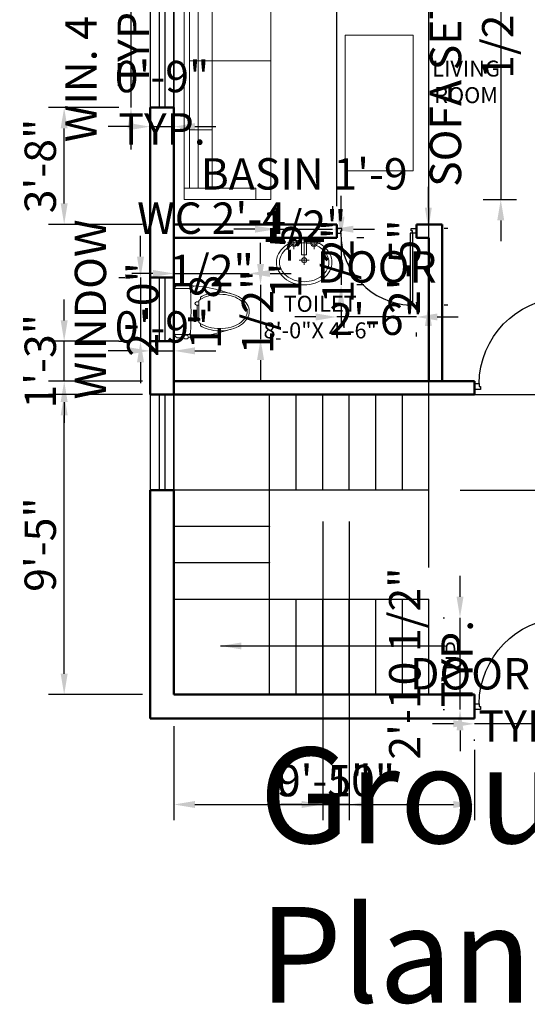
# Model space of a CAD drawing. Units: inches. Extents: x 117606 to 118050, y 251709 to 252357.
# Tile 1 of 3: x 117606 to 117797, y 251709 to 252079. Entities that reach past the tile are written whole.
import ezdxf

# ---------------------------------------------------------------- set-up
doc = ezdxf.new("R2010")
doc.units = ezdxf.units.IN
doc.header["$MEASUREMENT"] = 0
for name, color, linetype, lineweight in [('A-ANNO-SYMB', 7, 'Continuous', 18), ('A-ANNO-TEXT', 7, 'Continuous', 25), ('A-AREA-IDEN', 7, 'Continuous', 25), ('A-DOOR', 4, 'Continuous', 25), ('A-FLOR-CNST', 8, 'Continuous', 13), ('A-FLOR-STRS', 7, 'Continuous', 25), ('FURNITURE', 53, 'Continuous', 18), ('SANITARY', 151, 'Continuous', 18), ('WALL', 7, 'Continuous', 50), ('WINDOW', 2, 'Continuous', 25), ('YQ_DIM', 3, 'Continuous', 18)]:
    doc.layers.add(name, color=color, linetype=linetype, lineweight=lineweight)
doc.styles.add('YQ_DIM', font='SUPEROS.SHX', dxfattribs={"width": 0.8, "bigfont": 'HZDX.SHX'})
doc.dimstyles.new('yqi3_937', dxfattribs={"dimscale": 3.937008, "dimtxt": 3, "dimasz": 2, "dimexe": 1.5, "dimexo": 3, "dimgap": 0.5, "dimtad": 1, "dimdsep": 46, "dimlunit": 4, "dimtxsty": 'YQ_DIM', "dimcen": 0, "dimclrd": 256, "dimclre": 256, "dimclrt": 7, "dimadec": 1, "dimazin": 2, "dimtfac": 1, "dimtix": 1, "dimtmove": 2, "dimatfit": 2, "dimfxl": 1, "dimtolj": 1, "dimtzin": 0, "dimarcsym": 0})

# ---------------------------------------------------------------- blocks, each defined once
blk = doc.blocks.new('DR_D01')
for p, q in [((-0.45, 0.93), (-0.42, 0.93)), ((-0.45, 0.03), (-0.45, 0.93)), ((-0.42, 0.03), (-0.42, 0.93)), ((-0.5, 0.03), (-0.42, 0.03)), ((-0.5, 0.03), (-0.5, -0.03)), ((-0.45, 0.03), (-0.45, 0)), ((-0.45, 0), (-0.435, 0)), ((-0.435, 0), (-0.435, -0.03)), ((0.435, 0), (0.435, -0.03)), ((0.45, 0), (0.435, 0)), ((0.45, 0.03), (0.45, 0)), ((0.5, 0.03), (0.45, 0.03)), ((0.5, -0.03), (0.5, 0.03)), ((-0.435, -0.03), (-0.5, -0.03)), ((0.435, -0.03), (0.5, -0.03))]:
    blk.add_line(p, q)
blk.add_arc((-0.46, 0.021), 0.91, 0.5915, 87.4664)
blk = doc.blocks.new('WD_WIN4')
for p, q in [((-0.5, 0.5), (0.5, 0.5)), ((-0.5, 0.12), (0.5, 0.12)), ((-0.5, -0.12), (0.5, -0.12)), ((-0.5, -0.5), (0.5, -0.5))]:
    blk.add_line(p, q)
blk = doc.blocks.new('A$C4d06a8b4')
for p, q in [((27.06, 122.57), (27.06, 118.4)), ((27.06, 118.4), (0, 118.4)), ((2.07, 96.36), (2.07, 118.4)), ((5.25, 118.4), (5.25, 22.51)), ((10.59, 118.4), (10.59, 22.51)), ((10.59, 96.36), (2.07, 96.36)), ((2.07, 96.36), (2.07, 70.46)), ((2.07, 70.46), (10.59, 70.46)), ((2.07, 44.55), (2.07, 70.46)), ((10.59, 70.46), (32.66, 70.46)), ((10.59, 44.55), (2.07, 44.55)), ((2.07, 44.55), (2.07, 22.51)), ((27.06, 22.51), (0, 22.51)), ((27.06, 18.34), (27.06, 22.51)), ((42.51, 25.08), (38.34, 25.08)), ((42.51, 25.08), (42.51, 0)), ((96.71, 25.08), (96.71, 0)), ((96.71, 25.08), (100.88, 25.08)), ((42.51, 11.63), (96.71, 11.63)), ((96.71, 5.25), (42.51, 5.25)), ((42.51, 2.89), (96.71, 2.89))]:
    blk.add_line(p, q)
for points in [[(32.66, 122.57), (32.66, 18.34), (0, 18.34), (0, 122.57)], [(38.34, 0), (100.88, 0), (100.88, 32.66), (38.34, 32.66)]]:
    blk.add_lwpolyline(points, close=True)
at = {"color": 0, "linetype": 'ByBlock', "lineweight": -2}
blk.add_lwpolyline([(86.22, 60.81), (86.22, 111.84), (60.71, 111.84), (60.71, 60.81)], close=True, dxfattribs=at)
for points in [[(6.25, 16.33), (6.25, 34.21)], [(38.34, 16.33), (6.25, 16.33)]]:
    blk.add_lwpolyline(points, dxfattribs=at)
blk = doc.blocks.new('yq_matong_01')
for p, q in [((0, 200.5), (0, -200.5)), ((20, 220.5), (138.8, 220.5)), ((238, 104.1), (238, -104.1)), ((252.5, 138), (252.5, 114.5)), ((215.8, 91), (238, 91)), ((215.8, 61), (238, 61)), ((223, 61), (223, -61)), ((215.8, -61), (238, -61)), ((215.8, -91), (238, -91)), ((252.5, -114.5), (252.5, -138)), ((20, -220.5), (138.8, -220.5)), ((97.4, -220.5), (97.4, -225.5)), ((97.4, -225.5), (131.6, -225.5)), ((131.6, -220.5), (131.6, -225.5))]:
    blk.add_line(p, q)
for centre, radius, start, end in [((54.8, 202.4), 54.8, 117.32201, 181.89921), ((20, 200.5), 20, 90, 180), ((63.9, -1165.4), 1416.8, 71.40679, 91.38565), ((138.8, 200.5), 20, 2.30634, 90), ((216.6, 161.2), 83.2, 95.49628, 139.93242), ((-4840.4, 0), 5003.3, 357.69366, 2.30634), ((357.1, -47.5), 192.8, 123.27785, 128.13838), ((406.6, -122.9), 283, 105.20877, 123.27785), ((406.6, -122.9), 303, 105.20877, 120.56985), ((439, -242.2), 426.7, 74.79123, 105.20877), ((439, -242.2), 406.7, 74.79123, 105.20877), ((471.4, -122.9), 283, 56.72215, 74.79123), ((471.4, -122.9), 303, 56.72215, 74.79123), ((520.9, -47.5), 192.8, 32.25649, 56.72215), ((520.9, -47.5), 212.8, 32.25649, 56.72215), ((215.8, 76), 15, 90, 270), ((596.2, 0), 103.8, 360, 32.25649), ((596.2, 0), 123.8, 360, 32.25649), ((215.8, -76), 15, 90, 270), ((520.9, 47.5), 192.8, 303.27785, 327.74351), ((520.9, 47.5), 212.8, 303.27785, 327.74351), ((596.2, 0), 103.8, 327.74351, 360), ((596.2, 0), 123.8, 327.74351, 360), ((63.9, 1165.4), 1416.8, 272.89667, 288.59321), ((357.1, 47.5), 192.8, 231.86162, 236.72215), ((406.6, 122.9), 283, 236.72215, 254.79123), ((406.6, 122.9), 303, 239.43015, 254.79123), ((439, 242.2), 426.7, 254.79123, 285.20877), ((439, 242.2), 406.7, 254.79123, 285.20877), ((471.4, 122.9), 283, 285.20877, 303.27785), ((471.4, 122.9), 303, 285.20877, 303.27785), ((51.3, -204.4), 51.4, 175.68696, 245.09182), ((20, -200.5), 20, 180, 270), ((63.9, 1165.4), 1416.8, 268.61435, 271.20362), ((156.6, -247.4), 63.1, 159.68336, 188.49388), ((114.1, -225.6), 37, 237.52867, 304.27722), ((72.4, -247.4), 63.1, 352.09441, 20.31664), ((138.8, -200.5), 20, 270, 357.69366), ((216.6, -161.2), 83.2, 220.06758, 264.50372)]:
    blk.add_arc(centre, radius, start, end)
blk = doc.blocks.new('A$Ceac1d84d')
at = {"layer": 'SANITARY'}
blk.add_lwpolyline([(2.91, 20.31, 0.087396), (0.02, 1.17, 0.289473), (2, 0.01), (17.79, 0.01, 0.312446), (19.78, 1.17, 0.011298), (19.79, 3.69, 0.022445), (20.01, 3.71, 0.29977), (19.98, 5.32, 0.02582), (19.73, 5.34, 0.068596), (16.89, 20.31, 0.021224), (16.57, 21.7, 0.079005), (15.03, 25.11, 0.107159), (12.5, 27.6, 0.141682), (9.9, 28.35, 0.141682), (7.3, 27.6, 0.107159), (4.76, 25.11, 0.079005), (3.23, 21.7, 0.021224)], format="xyb", close=True, dxfattribs=at)
at = {"layer": 'SANITARY', "xscale": 0.0393700787401575, "yscale": 0.0393700787401575, "zscale": 0.0393700787401575, "rotation": 89.99999999999407}
blk.add_blockref('yq_matong_01', (9.9, 0.01), dxfattribs=at)
blk = doc.blocks.new('yq_sink_01')
for p, q in [((130.9, 96.8), (25.6, 96.8)), ((69.5, 23.9), (69.5, 157.9)), ((182.6, 23.9), (20, 23.9)), ((20, 23.9), (20, -23.9)), ((182.6, 23.9), (182.5, -24)), ((235.6, 47.8), (235.6, -47.9)), ((182.5, -24), (20, -23.9)), ((278.3, -0.1), (25.5, 0)), ((69.4, -24), (69.4, -157.9)), ((130.8, -96.9), (25.5, -96.8))]:
    blk.add_line(p, q)
for centre, radius in [((69.5, 95.2), 33.5), ((69.5, 95.2), 23.9), ((235.6, 0.6), 23.9), ((69.4, -95.2), 33.5), ((69.4, -95.2), 23.9)]:
    blk.add_circle(centre, radius)
for centre, radius, start, end in [((312, 19.4), 268.6, 140.95411, 156.02098), ((277.5, 47.4), 224.1, 117.05223, 140.95411), ((277.5, 47.4), 194.7, 117.05223, 140.95411), ((255.4, 90.6), 175.7, 62.94777, 117.05223), ((255.4, 90.6), 146.2, 62.94777, 117.05223), ((233.4, 47.4), 194.7, 39.04589, 62.94777), ((233.4, 47.4), 224.1, 39.04589, 62.94777), ((198.8, 19.4), 268.6, 18.57097, 39.04589), ((312, 19.4), 239.1, 140.95411, 155.66772), ((198.8, 19.4), 239.1, 18.57097, 39.04589), ((144.5, 1.2), 296.4, 0, 18.57097), ((144.5, 1.2), 325.9, 360, 18.57097), ((366.3, 1.2), 325.9, 167.86118, 192.49263), ((366.3, 1.2), 296.4, 168.09162, 192.40027), ((144.5, 1.2), 296.4, 341.42903, 360), ((144.5, 1.2), 325.9, 341.42903, 360), ((198.8, -17.1), 239.1, 320.95411, 341.42903), ((312, -17.1), 268.6, 204.55072, 219.04589), ((312, -17.1), 239.1, 204.73595, 219.04589), ((277.5, -45.1), 224.1, 219.04589, 242.94777), ((277.5, -45.1), 194.7, 219.04589, 242.94777), ((233.4, -45.1), 194.7, 297.05223, 320.95411), ((233.4, -45.1), 224.1, 297.05223, 320.95411), ((198.8, -17.1), 268.6, 320.95411, 341.42903), ((255.4, -88.2), 175.7, 242.94777, 297.05223), ((255.4, -88.2), 146.2, 242.94777, 297.05223)]:
    blk.add_arc(centre, radius, start, end)
blk = doc.blocks.new('*D141')
at = {"layer": 'Defpoints', "color": 0, "transparency": 16777216}
for p in [(117654.89, 252094.28), (117647.69, 252046.28), (117654.89, 252046.28)]:
    blk.add_point(p, dxfattribs=at)
at = {"layer": 'YQ_DIM', "lineweight": -2, "transparency": 16777216}
for p, q in [((117647.69, 252102.16), (117647.69, 252110.03)), ((117643.07, 252094.28), (117641.78, 252094.28)), ((117647.69, 252094.28), (117647.69, 252046.28)), ((117643.07, 252046.28), (117641.78, 252046.28)), ((117647.69, 252038.41), (117647.69, 252030.54))]:
    blk.add_line(p, q, dxfattribs=at)
at = {"layer": 'YQ_DIM', "transparency": 16777216}
for points in [[(117646.37, 252102.16), (117649, 252102.16), (117647.69, 252094.28)], [(117646.37, 252038.41), (117649, 252038.41), (117647.69, 252046.28)]]:
    blk.add_solid(points, dxfattribs=at)
at = {"layer": 'YQ_DIM', "color": 7, "transparency": 16777216, "insert": (117638.69, 252070.28), "char_height": 11.811, "attachment_point": 5, "rotation": 90, "style": 'YQ_DIM'}
blk.add_mtext('\\A1;WIN. 4\'-0" TYP.', dxfattribs=at)
blk = doc.blocks.new('*D142')
at = {"layer": 'Defpoints', "color": 0, "transparency": 16777216}
for p in [(117654.89, 252046.28), (117663.89, 252046.28), (117663.89, 252039.08)]:
    blk.add_point(p, dxfattribs=at)
at = {"layer": 'YQ_DIM', "lineweight": -2, "transparency": 16777216}
for p, q in [((117647.01, 252039.08), (117639.14, 252039.08)), ((117654.89, 252039.08), (117663.89, 252039.08)), ((117671.76, 252039.08), (117679.63, 252039.08)), ((117654.89, 252034.47), (117654.89, 252033.18)), ((117663.89, 252034.47), (117663.89, 252033.18))]:
    blk.add_line(p, q, dxfattribs=at)
at = {"layer": 'YQ_DIM', "transparency": 16777216}
for points in [[(117647.01, 252040.4), (117647.01, 252037.77), (117654.89, 252039.08)], [(117671.76, 252040.4), (117671.76, 252037.77), (117663.89, 252039.08)]]:
    blk.add_solid(points, dxfattribs=at)
at = {"layer": 'YQ_DIM', "color": 7, "transparency": 16777216, "insert": (117659.39, 252048.08), "char_height": 11.811, "attachment_point": 5, "style": 'YQ_DIM'}
blk.add_mtext('\\A1;0\'-9" TYP.', dxfattribs=at)
blk = doc.blocks.new('*D145')
at = {"layer": 'Defpoints', "color": 0, "transparency": 16777216}
for p in [(117654.89, 251982.28), (117651.29, 251958.28), (117654.89, 251958.28)]:
    blk.add_point(p, dxfattribs=at)
at = {"layer": 'YQ_DIM', "lineweight": -2, "transparency": 16777216}
for p, q in [((117651.29, 251990.16), (117651.29, 251998.03)), ((117643.07, 251982.28), (117645.38, 251982.28)), ((117651.29, 251982.28), (117651.29, 251958.28)), ((117643.07, 251958.28), (117645.38, 251958.28)), ((117651.29, 251950.41), (117651.29, 251942.54))]:
    blk.add_line(p, q, dxfattribs=at)
at = {"layer": 'YQ_DIM', "transparency": 16777216}
for points in [[(117649.97, 251990.16), (117652.6, 251990.16), (117651.29, 251982.28)], [(117649.97, 251950.41), (117652.6, 251950.41), (117651.29, 251958.28)]]:
    blk.add_solid(points, dxfattribs=at)
at = {"layer": 'YQ_DIM', "color": 7, "transparency": 16777216, "insert": (117642.29, 251970.28), "char_height": 11.811, "attachment_point": 5, "rotation": 90, "style": 'YQ_DIM'}
blk.add_mtext('\\A1;WINDOW 2\'-0"', dxfattribs=at)
blk = doc.blocks.new('*D146')
at = {"layer": 'Defpoints', "color": 0, "transparency": 16777216}
for p in [(117654.89, 251958.28), (117663.89, 251958.28), (117663.89, 251954.68)]:
    blk.add_point(p, dxfattribs=at)
at = {"layer": 'YQ_DIM', "lineweight": -2, "transparency": 16777216}
for p, q in [((117647.01, 251954.68), (117639.14, 251954.68)), ((117654.89, 251954.68), (117663.89, 251954.68)), ((117671.76, 251954.68), (117679.63, 251954.68)), ((117654.89, 251946.47), (117654.89, 251948.78)), ((117663.89, 251946.47), (117663.89, 251948.78))]:
    blk.add_line(p, q, dxfattribs=at)
at = {"layer": 'YQ_DIM', "transparency": 16777216}
for points in [[(117647.01, 251956), (117647.01, 251953.37), (117654.89, 251954.68)], [(117671.76, 251956), (117671.76, 251953.37), (117663.89, 251954.68)]]:
    blk.add_solid(points, dxfattribs=at)
at = {"layer": 'YQ_DIM', "color": 7, "transparency": 16777216, "insert": (117659.39, 251963.68), "char_height": 11.811, "attachment_point": 5, "style": 'YQ_DIM'}
blk.add_mtext('\\A1;0\'-9"', dxfattribs=at)
blk = doc.blocks.new('*D147')
at = {"layer": 'Defpoints', "color": 0, "transparency": 16777216}
for p in [(117777.01, 251819.7), (117813.01, 251819.7), (117777.01, 251814.3)]:
    blk.add_point(p, dxfattribs=at)
at = {"layer": 'YQ_DIM', "lineweight": -2, "transparency": 16777216}
for p, q in [((117769.14, 251814.3), (117761.26, 251814.3)), ((117813.01, 251814.3), (117777.01, 251814.3)), ((117820.89, 251814.3), (117828.76, 251814.3)), ((117777.01, 251807.89), (117777.01, 251808.4)), ((117813.01, 251807.89), (117813.01, 251808.4))]:
    blk.add_line(p, q, dxfattribs=at)
at = {"layer": 'YQ_DIM', "transparency": 16777216}
for points in [[(117769.14, 251815.62), (117769.14, 251812.99), (117777.01, 251814.3)], [(117820.89, 251815.62), (117820.89, 251812.99), (117813.01, 251814.3)]]:
    blk.add_solid(points, dxfattribs=at)
at = {"layer": 'YQ_DIM', "color": 7, "transparency": 16777216, "insert": (117795.01, 251823.3), "char_height": 11.811, "attachment_point": 5, "style": 'YQ_DIM'}
blk.add_mtext('\\A1;DOOR 3\'-0" TYP.', dxfattribs=at)
blk = doc.blocks.new('*D148')
at = {"layer": 'Defpoints', "color": 0, "transparency": 16777216}
for p in [(117771.61, 251854.26), (117777.01, 251854.26), (117777.01, 251819.7)]:
    blk.add_point(p, dxfattribs=at)
at = {"layer": 'YQ_DIM', "lineweight": -2, "transparency": 16777216}
for p, q in [((117771.61, 251862.14), (117771.61, 251870.01)), ((117765.2, 251854.26), (117765.71, 251854.26)), ((117771.61, 251819.7), (117771.61, 251854.26)), ((117765.2, 251819.7), (117765.71, 251819.7)), ((117771.61, 251811.83), (117771.61, 251803.96))]:
    blk.add_line(p, q, dxfattribs=at)
at = {"layer": 'YQ_DIM', "transparency": 16777216}
for points in [[(117770.3, 251862.14), (117772.92, 251862.14), (117771.61, 251854.26)], [(117770.3, 251811.83), (117772.92, 251811.83), (117771.61, 251819.7)]]:
    blk.add_solid(points, dxfattribs=at)
at = {"layer": 'YQ_DIM', "color": 7, "transparency": 16777216, "insert": (117760.64, 251836.98), "char_height": 11.811, "attachment_point": 5, "rotation": 90, "style": 'YQ_DIM'}
blk.add_mtext('\\A1;2\'-10 1/2" TYP.', dxfattribs=at)
blk = doc.blocks.new('*D149')
at = {"layer": 'Defpoints', "color": 0, "transparency": 16777216}
for p in [(117725.19, 251971.94), (117755.19, 251971.94), (117725.19, 251967.44)]:
    blk.add_point(p, dxfattribs=at)
at = {"layer": 'YQ_DIM', "lineweight": -2, "transparency": 16777216}
for p, q in [((117717.31, 251967.44), (117709.44, 251967.44)), ((117755.19, 251967.44), (117725.19, 251967.44)), ((117763.06, 251967.44), (117770.94, 251967.44)), ((117725.19, 251960.13), (117725.19, 251961.54)), ((117755.19, 251960.13), (117755.19, 251961.54))]:
    blk.add_line(p, q, dxfattribs=at)
at = {"layer": 'YQ_DIM', "transparency": 16777216}
for points in [[(117717.31, 251968.76), (117717.31, 251966.13), (117725.19, 251967.44)], [(117763.06, 251968.76), (117763.06, 251966.13), (117755.19, 251967.44)]]:
    blk.add_solid(points, dxfattribs=at)
at = {"layer": 'YQ_DIM', "color": 7, "transparency": 16777216, "insert": (117740.19, 251976.44), "char_height": 11.811, "attachment_point": 5, "style": 'YQ_DIM'}
blk.add_mtext('\\A1;DOOR 2\'-6"', dxfattribs=at)
blk = doc.blocks.new('*D150')
at = {"layer": 'Defpoints', "color": 0, "transparency": 16777216}
for p in [(117755.19, 252000.74), (117755.19, 251971.94), (117759.69, 251971.94)]:
    blk.add_point(p, dxfattribs=at)
at = {"layer": 'YQ_DIM', "lineweight": -2, "transparency": 16777216}
for p, q in [((117759.69, 252008.62), (117759.69, 252016.49)), ((117759.69, 252000.74), (117759.69, 251971.94)), ((117767, 252000.74), (117765.59, 252000.74)), ((117767, 251971.94), (117765.59, 251971.94)), ((117759.69, 251964.07), (117759.69, 251956.2))]:
    blk.add_line(p, q, dxfattribs=at)
at = {"layer": 'YQ_DIM', "transparency": 16777216}
for points in [[(117758.38, 252008.62), (117761, 252008.62), (117759.69, 252000.74)], [(117758.38, 251964.07), (117761, 251964.07), (117759.69, 251971.94)]]:
    blk.add_solid(points, dxfattribs=at)
at = {"layer": 'YQ_DIM', "color": 7, "transparency": 16777216, "insert": (117750.69, 251986.34), "char_height": 11.811, "attachment_point": 5, "rotation": 90, "style": 'YQ_DIM'}
blk.add_mtext('\\A1;2\'-5"', dxfattribs=at)
blk = doc.blocks.new('*D159')
at = {"layer": 'Defpoints', "color": 0, "transparency": 16777216}
for p in [(117768.57, 252134.27), (117768.57, 252011.7), (117786.95, 252011.7)]:
    blk.add_point(p, dxfattribs=at)
at = {"layer": 'YQ_DIM', "lineweight": -2, "transparency": 16777216}
for p, q in [((117786.95, 252142.14), (117786.95, 252150.02)), ((117780.38, 252134.27), (117792.86, 252134.27)), ((117786.95, 252134.27), (117786.95, 252011.7)), ((117780.38, 252011.7), (117792.86, 252011.7)), ((117786.95, 252003.82), (117786.95, 251995.95))]:
    blk.add_line(p, q, dxfattribs=at)
at = {"layer": 'YQ_DIM', "transparency": 16777216}
for points in [[(117785.64, 252142.14), (117788.26, 252142.14), (117786.95, 252134.27)], [(117785.64, 252003.82), (117788.26, 252003.82), (117786.95, 252011.7)]]:
    blk.add_solid(points, dxfattribs=at)
at = {"layer": 'YQ_DIM', "color": 7, "transparency": 16777216, "insert": (117775.98, 252072.98), "char_height": 11.811, "attachment_point": 5, "rotation": 90, "style": 'YQ_DIM'}
blk.add_mtext('\\A1;SOFA SET 10\'-2 1/2"', dxfattribs=at)
blk = doc.blocks.new('*D161')
at = {"layer": 'Defpoints', "color": 0, "transparency": 16777216}
for p in [(117723.61, 252000.49), (117702.23, 251997.28), (117723.61, 251997.28)]:
    blk.add_point(p, dxfattribs=at)
at = {"layer": 'YQ_DIM', "lineweight": -2, "transparency": 16777216}
for p, q in [((117702.23, 252009.1), (117702.23, 252006.4)), ((117723.61, 252009.1), (117723.61, 252006.4)), ((117694.36, 252000.49), (117686.48, 252000.49)), ((117702.23, 252000.49), (117723.61, 252000.49)), ((117731.48, 252000.49), (117739.36, 252000.49))]:
    blk.add_line(p, q, dxfattribs=at)
at = {"layer": 'YQ_DIM', "transparency": 16777216}
for points in [[(117694.36, 252001.8), (117694.36, 251999.18), (117702.23, 252000.49)], [(117731.48, 252001.8), (117731.48, 251999.18), (117723.61, 252000.49)]]:
    blk.add_solid(points, dxfattribs=at)
at = {"layer": 'YQ_DIM', "color": 7, "transparency": 16777216, "insert": (117712.92, 252011.46), "char_height": 11.811, "attachment_point": 5, "style": 'YQ_DIM'}
blk.add_mtext('\\A1;BASIN 1\'-9 1/2"', dxfattribs=at)
blk = doc.blocks.new('*D162')
at = {"layer": 'Defpoints', "color": 0, "transparency": 16777216}
for p in [(117723.61, 251997.28), (117723.61, 251979.55), (117726.82, 251979.55)]:
    blk.add_point(p, dxfattribs=at)
at = {"layer": 'YQ_DIM', "lineweight": -2, "transparency": 16777216}
for p, q in [((117726.82, 252005.16), (117726.82, 252013.03)), ((117726.82, 251997.28), (117726.82, 251979.55)), ((117735.42, 251997.28), (117732.72, 251997.28)), ((117735.42, 251979.55), (117732.72, 251979.55)), ((117726.82, 251971.68), (117726.82, 251963.8))]:
    blk.add_line(p, q, dxfattribs=at)
at = {"layer": 'YQ_DIM', "transparency": 16777216}
for points in [[(117725.51, 252005.16), (117728.13, 252005.16), (117726.82, 251997.28)], [(117725.51, 251971.68), (117728.13, 251971.68), (117726.82, 251979.55)]]:
    blk.add_solid(points, dxfattribs=at)
at = {"layer": 'YQ_DIM', "color": 7, "transparency": 16777216, "insert": (117715.85, 251988.42), "char_height": 11.811, "attachment_point": 5, "rotation": 90, "style": 'YQ_DIM'}
blk.add_mtext('\\A1;1\'-5 1/2"', dxfattribs=at)
blk = doc.blocks.new('*D163')
at = {"layer": 'Defpoints', "color": 0, "transparency": 16777216}
for p in [(117692.23, 251983.82), (117663.82, 251979.56), (117692.23, 251979.56)]:
    blk.add_point(p, dxfattribs=at)
at = {"layer": 'YQ_DIM', "lineweight": -2, "transparency": 16777216}
for p, q in [((117663.82, 251991.37), (117663.82, 251989.73)), ((117692.23, 251991.37), (117692.23, 251989.73)), ((117655.95, 251983.82), (117648.07, 251983.82)), ((117663.82, 251983.82), (117692.23, 251983.82)), ((117700.11, 251983.82), (117707.98, 251983.82))]:
    blk.add_line(p, q, dxfattribs=at)
at = {"layer": 'YQ_DIM', "transparency": 16777216}
for points in [[(117655.95, 251985.13), (117655.95, 251982.51), (117663.82, 251983.82)], [(117700.11, 251985.13), (117700.11, 251982.51), (117692.23, 251983.82)]]:
    blk.add_solid(points, dxfattribs=at)
at = {"layer": 'YQ_DIM', "color": 7, "transparency": 16777216, "insert": (117678.03, 251994.79), "char_height": 11.811, "attachment_point": 5, "style": 'YQ_DIM'}
blk.add_mtext('\\A1;WC 2\'-4 1/2"', dxfattribs=at)
blk = doc.blocks.new('*D164')
at = {"layer": 'Defpoints', "color": 0, "transparency": 16777216}
for p in [(117692.23, 251979.56), (117692.23, 251959.1), (117696.49, 251959.1)]:
    blk.add_point(p, dxfattribs=at)
at = {"layer": 'YQ_DIM', "lineweight": -2, "transparency": 16777216}
for p, q in [((117696.49, 251987.43), (117696.49, 251995.31)), ((117696.49, 251979.56), (117696.49, 251959.1)), ((117704.04, 251979.56), (117702.4, 251979.56)), ((117704.04, 251959.1), (117702.4, 251959.1)), ((117696.49, 251951.22), (117696.49, 251943.35))]:
    blk.add_line(p, q, dxfattribs=at)
at = {"layer": 'YQ_DIM', "transparency": 16777216}
for points in [[(117695.18, 251987.43), (117697.81, 251987.43), (117696.49, 251979.56)], [(117695.18, 251951.22), (117697.81, 251951.22), (117696.49, 251959.1)]]:
    blk.add_solid(points, dxfattribs=at)
at = {"layer": 'YQ_DIM', "color": 7, "transparency": 16777216, "insert": (117685.53, 251969.33), "char_height": 11.811, "attachment_point": 5, "rotation": 90, "style": 'YQ_DIM'}
blk.add_mtext('\\A1;1\'-8 1/2"', dxfattribs=at)
blk = doc.blocks.new('*D166')
at = {"layer": 'Defpoints', "color": 0, "transparency": 16777216}
for p in [(117622.54, 251938.28), (117663.89, 251938.28), (117663.89, 251825.28)]:
    blk.add_point(p, dxfattribs=at)
at = {"layer": 'YQ_DIM', "lineweight": -2, "transparency": 16777216}
for p, q in [((117652.07, 251938.28), (117616.63, 251938.28)), ((117622.54, 251833.16), (117622.54, 251930.41)), ((117652.07, 251825.28), (117616.63, 251825.28))]:
    blk.add_line(p, q, dxfattribs=at)
at = {"layer": 'YQ_DIM', "transparency": 16777216}
for points in [[(117621.22, 251930.41), (117623.85, 251930.41), (117622.54, 251938.28)], [(117621.22, 251833.16), (117623.85, 251833.16), (117622.54, 251825.28)]]:
    blk.add_solid(points, dxfattribs=at)
at = {"layer": 'YQ_DIM', "color": 7, "transparency": 16777216, "insert": (117613.54, 251881.78), "char_height": 11.811, "attachment_point": 5, "rotation": 90, "style": 'YQ_DIM'}
blk.add_mtext('\\A1;9\'-5"', dxfattribs=at)
blk = doc.blocks.new('*D168')
at = {"layer": 'Defpoints', "color": 0, "transparency": 16777216}
for p in [(117759.89, 252328.63), (117663.89, 251861.28), (117759.89, 251861.28)]:
    blk.add_point(p, dxfattribs=at)
at = {"layer": 'YQ_DIM', "lineweight": -2, "transparency": 16777216}
for p, q in [((117663.89, 251873.1), (117663.89, 252334.54)), ((117759.89, 251873.1), (117759.89, 252334.54)), ((117671.76, 252328.63), (117752.01, 252328.63))]:
    blk.add_line(p, q, dxfattribs=at)
at = {"layer": 'YQ_DIM', "transparency": 16777216}
for points in [[(117671.76, 252329.95), (117671.76, 252327.32), (117663.89, 252328.63)], [(117752.01, 252329.95), (117752.01, 252327.32), (117759.89, 252328.63)]]:
    blk.add_solid(points, dxfattribs=at)
at = {"layer": 'YQ_DIM', "color": 7, "transparency": 16777216, "insert": (117711.89, 252337.63), "char_height": 11.811, "attachment_point": 5, "style": 'YQ_DIM'}
blk.add_mtext('\\A1;8\'-0"', dxfattribs=at)
blk = doc.blocks.new('*D169')
at = {"layer": 'Defpoints', "color": 0, "transparency": 16777216}
for p in [(117759.89, 251938.28), (117759.89, 251902.28), (118011.24, 251902.28)]:
    blk.add_point(p, dxfattribs=at)
at = {"layer": 'YQ_DIM', "lineweight": -2, "transparency": 16777216}
for p, q in [((118011.24, 251946.16), (118011.24, 251954.03)), ((117771.7, 251938.28), (118017.14, 251938.28)), ((118011.24, 251938.28), (118011.24, 251902.28)), ((117771.7, 251902.28), (118017.14, 251902.28)), ((118011.24, 251894.41), (118011.24, 251886.54))]:
    blk.add_line(p, q, dxfattribs=at)
at = {"layer": 'YQ_DIM', "transparency": 16777216}
for points in [[(118009.92, 251946.16), (118012.55, 251946.16), (118011.24, 251938.28)], [(118009.92, 251894.41), (118012.55, 251894.41), (118011.24, 251902.28)]]:
    blk.add_solid(points, dxfattribs=at)
at = {"layer": 'YQ_DIM', "color": 7, "transparency": 16777216, "insert": (118002.24, 251920.28), "char_height": 11.811, "attachment_point": 5, "rotation": 90, "style": 'YQ_DIM'}
blk.add_mtext('\\A1;3\'-0"', dxfattribs=at)
blk = doc.blocks.new('*D170')
at = {"layer": 'Defpoints', "color": 0, "transparency": 16777216}
for p in [(117719.89, 251902.28), (117729.89, 251902.28), (117719.89, 251783.93)]:
    blk.add_point(p, dxfattribs=at)
at = {"layer": 'YQ_DIM', "lineweight": -2, "transparency": 16777216}
for p, q in [((117719.89, 251890.47), (117719.89, 251778.03)), ((117729.89, 251890.47), (117729.89, 251778.03)), ((117712.01, 251783.93), (117704.14, 251783.93)), ((117729.89, 251783.93), (117719.89, 251783.93)), ((117737.76, 251783.93), (117745.63, 251783.93))]:
    blk.add_line(p, q, dxfattribs=at)
at = {"layer": 'YQ_DIM', "transparency": 16777216}
for points in [[(117712.01, 251785.25), (117712.01, 251782.62), (117719.89, 251783.93)], [(117737.76, 251785.25), (117737.76, 251782.62), (117729.89, 251783.93)]]:
    blk.add_solid(points, dxfattribs=at)
at = {"layer": 'YQ_DIM', "color": 7, "transparency": 16777216, "insert": (117724.89, 251792.93), "char_height": 11.811, "attachment_point": 5, "style": 'YQ_DIM'}
blk.add_mtext('\\A1;0\'-10"', dxfattribs=at)
blk = doc.blocks.new('*D171')
at = {"layer": 'Defpoints', "color": 0, "transparency": 16777216}
for p in [(117663.89, 251825.28), (117777.01, 251816.28), (117777.01, 251783.93)]:
    blk.add_point(p, dxfattribs=at)
at = {"layer": 'YQ_DIM', "lineweight": -2, "transparency": 16777216}
for p, q in [((117663.89, 251813.47), (117663.89, 251778.03)), ((117777.01, 251804.47), (117777.01, 251778.03)), ((117671.76, 251783.93), (117769.14, 251783.93))]:
    blk.add_line(p, q, dxfattribs=at)
at = {"layer": 'YQ_DIM', "transparency": 16777216}
for points in [[(117671.76, 251785.25), (117671.76, 251782.62), (117663.89, 251783.93)], [(117769.14, 251785.25), (117769.14, 251782.62), (117777.01, 251783.93)]]:
    blk.add_solid(points, dxfattribs=at)
at = {"layer": 'YQ_DIM', "color": 7, "transparency": 16777216, "insert": (117720.45, 251792.93), "char_height": 11.811, "attachment_point": 5, "style": 'YQ_DIM'}
blk.add_mtext('\\A1;9\'-5"', dxfattribs=at)
blk = doc.blocks.new('*D176')
at = {"layer": 'Defpoints', "color": 0, "transparency": 16777216}
for p in [(117622.54, 252046.28), (117654.89, 252046.28), (117663.89, 252002.28)]:
    blk.add_point(p, dxfattribs=at)
at = {"layer": 'YQ_DIM', "lineweight": -2, "transparency": 16777216}
for p, q in [((117643.07, 252046.28), (117616.63, 252046.28)), ((117622.54, 252010.16), (117622.54, 252038.41)), ((117652.07, 252002.28), (117616.63, 252002.28))]:
    blk.add_line(p, q, dxfattribs=at)
at = {"layer": 'YQ_DIM', "transparency": 16777216}
for points in [[(117621.22, 252038.41), (117623.85, 252038.41), (117622.54, 252046.28)], [(117621.22, 252010.16), (117623.85, 252010.16), (117622.54, 252002.28)]]:
    blk.add_solid(points, dxfattribs=at)
at = {"layer": 'YQ_DIM', "color": 7, "transparency": 16777216, "insert": (117613.54, 252024.28), "char_height": 11.811, "attachment_point": 5, "rotation": 90, "style": 'YQ_DIM'}
blk.add_mtext('\\A1;3\'-8"', dxfattribs=at)
blk = doc.blocks.new('*D177')
at = {"layer": 'Defpoints', "color": 0, "transparency": 16777216}
for p in [(117622.54, 251958.28), (117654.89, 251958.28), (117663.89, 251943.28)]:
    blk.add_point(p, dxfattribs=at)
at = {"layer": 'YQ_DIM', "lineweight": -2, "transparency": 16777216}
for p, q in [((117622.54, 251966.16), (117622.54, 251974.03)), ((117643.07, 251958.28), (117616.63, 251958.28)), ((117622.54, 251943.28), (117622.54, 251958.28)), ((117652.07, 251943.28), (117616.63, 251943.28)), ((117622.54, 251935.41), (117622.54, 251927.54))]:
    blk.add_line(p, q, dxfattribs=at)
at = {"layer": 'YQ_DIM', "transparency": 16777216}
for points in [[(117621.22, 251966.16), (117623.85, 251966.16), (117622.54, 251958.28)], [(117621.22, 251935.41), (117623.85, 251935.41), (117622.54, 251943.28)]]:
    blk.add_solid(points, dxfattribs=at)
at = {"layer": 'YQ_DIM', "color": 7, "transparency": 16777216, "insert": (117613.54, 251950.78), "char_height": 11.811, "attachment_point": 5, "rotation": 90, "style": 'YQ_DIM'}
blk.add_mtext('\\A1;1\'-3"', dxfattribs=at)
blk = doc.blocks.new('*D180')
at = {"layer": 'Defpoints', "color": 0, "transparency": 16777216}
for p in [(117725.19, 252328.63), (117663.89, 251997.28), (117725.19, 251997.28)]:
    blk.add_point(p, dxfattribs=at)
at = {"layer": 'YQ_DIM', "lineweight": -2, "transparency": 16777216}
for p, q in [((117663.89, 252009.1), (117663.89, 252334.54)), ((117725.19, 252009.1), (117725.19, 252334.54)), ((117656.01, 252328.63), (117648.14, 252328.63)), ((117663.89, 252328.63), (117725.19, 252328.63)), ((117733.06, 252328.63), (117740.94, 252328.63))]:
    blk.add_line(p, q, dxfattribs=at)
at = {"layer": 'YQ_DIM', "transparency": 16777216}
for points in [[(117656.01, 252329.95), (117656.01, 252327.32), (117663.89, 252328.63)], [(117733.06, 252329.95), (117733.06, 252327.32), (117725.19, 252328.63)]]:
    blk.add_solid(points, dxfattribs=at)
at = {"layer": 'YQ_DIM', "color": 7, "transparency": 16777216, "insert": (117694.54, 252339.6), "char_height": 11.811, "attachment_point": 5, "style": 'YQ_DIM'}
blk.add_mtext('\\A1;5\'-1 1/2"', dxfattribs=at)

msp = doc.modelspace()

# ---------------------------------------------------------------- linework, layer by layer
at = {"layer": 'A-FLOR-CNST'}
for p in [(117699.885, 251888.617), (117699.885, 251874.951)]:
    msp.add_point(p, dxfattribs=at)
at = {"layer": 'A-FLOR-STRS'}
for p, q in [((117699.885, 251902.284), (117699.885, 251938.284)), ((117709.885, 251902.284), (117709.885, 251938.284)), ((117719.885, 251902.284), (117719.885, 251938.284)), ((117729.885, 251902.284), (117729.885, 251938.284)), ((117739.885, 251902.284), (117739.885, 251938.284)), ((117749.885, 251902.284), (117749.885, 251938.284)), ((117759.885, 251902.284), (117759.885, 251938.284)), ((117699.885, 251902.284), (117663.885, 251902.284)), ((117759.885, 251902.284), (117699.885, 251902.284)), ((117699.885, 251861.284), (117699.885, 251902.284)), ((117699.885, 251888.617), (117663.885, 251888.617)), ((117699.885, 251874.951), (117663.885, 251874.951)), ((117663.885, 251861.284), (117759.885, 251861.284)), ((117699.885, 251825.284), (117699.885, 251861.284)), ((117709.885, 251825.284), (117709.885, 251861.284)), ((117719.885, 251825.284), (117719.885, 251861.284)), ((117729.885, 251825.284), (117729.885, 251861.284)), ((117739.885, 251825.284), (117739.885, 251861.284)), ((117749.885, 251825.284), (117749.885, 251861.284)), ((117759.885, 251825.284), (117759.885, 251861.284))]:
    msp.add_line(p, q, dxfattribs=at)
at = {"layer": 'WALL'}
for p, q in [((117663.885, 252046.284), (117654.885, 252046.284)), ((117654.885, 251938.284), (117654.885, 252046.284)), ((117663.885, 251997.284), (117663.885, 252046.284)), ((117725.188, 252002.284), (117663.885, 252002.284)), ((117725.188, 251997.284), (117725.188, 252002.284)), ((117764.885, 252002.284), (117755.188, 252002.284)), ((117755.188, 251997.284), (117755.188, 252002.284)), ((117764.885, 251943.284), (117764.885, 252002.284)), ((117663.885, 251943.284), (117663.885, 251997.284)), ((117725.188, 251997.284), (117663.885, 251997.284)), ((117759.885, 251997.284), (117755.188, 251997.284)), ((117759.885, 251943.284), (117759.885, 251997.284)), ((117663.885, 251982.284), (117654.885, 251982.284)), ((117654.885, 251958.284), (117663.885, 251958.284)), ((117777.031, 251943.284), (117663.885, 251943.284)), ((117663.885, 251938.284), (117663.885, 251943.284)), ((117777.031, 251943.284), (117777.031, 251938.284)), ((117663.885, 251938.284), (117654.885, 251938.284)), ((117777.031, 251938.284), (117663.885, 251938.284)), ((117654.885, 251816.284), (117654.885, 251902.284)), ((117663.885, 251902.284), (117654.885, 251902.284)), ((117663.885, 251825.284), (117663.885, 251902.284)), ((117663.885, 251825.284), (117777.011, 251825.284)), ((117777.011, 251825.284), (117777.011, 251816.284)), ((117654.885, 251816.284), (117777.011, 251816.284))]:
    msp.add_line(p, q, dxfattribs=at)

# ---------------------------------------------------------------- block references
at = {"layer": 'A-DOOR', "rotation": 180}
for p, xscale, yscale, zscale in [((117740.188, 251999.845), 30, 30, 30), ((117795.011, 251941.28), 36, -36, 36), ((117795.011, 251820.784), 36, -36, 36)]:
    msp.add_blockref('DR_D01', p, dxfattribs=dict(at, xscale=xscale, yscale=yscale, zscale=zscale))
at = {"layer": 'FURNITURE', "xscale": -1, "rotation": 180}
msp.add_blockref('A$C4d06a8b4', (117667.688, 252134.269), dxfattribs=at)
at = {"layer": 'SANITARY', "xscale": 0.0393700787401575, "yscale": 0.0393700787401575, "zscale": 0.0393700787401575, "rotation": 269.999999999994}
msp.add_blockref('yq_sink_01', (117712.876, 251998.071), dxfattribs=at)
at = {"layer": 'SANITARY', "rotation": 270}
msp.add_blockref('A$Ceac1d84d', (117663.88, 251979.417), dxfattribs=at)
at = {"layer": 'WINDOW'}
for p, xscale, yscale, zscale, rotation in [((117659.385, 252070.284), 48, 9.000000000043656, 48, 269.9999999999826), ((117659.385, 251970.284), 24, 9, 24, 270), ((117659.385, 251920.284), 36, 9.000000000029104, 36, 269.9999999999769)]:
    msp.add_blockref('WD_WIN4', p, dxfattribs=dict(at, xscale=xscale, yscale=yscale, zscale=zscale, rotation=rotation))

# ---------------------------------------------------------------- texts
at = {"layer": 'A-ANNO-TEXT', "insert": (117766.184, 251836.15), "char_height": 6, "width": 7.46712, "attachment_point": 1, "rotation": 90, "style": 'YQ_DIM'}
msp.add_mtext('\\pxqc;UP', dxfattribs=at)
at = {"layer": 'A-ANNO-TEXT', "insert": (117696.03, 251805.364), "char_height": 36, "width": 336.12923, "attachment_point": 1, "style": 'YQ_DIM'}
msp.add_mtext('Ground Floor Plan', dxfattribs=at)
at = {"layer": 'A-AREA-IDEN', "char_height": 6, "attachment_point": 1, "style": 'YQ_DIM'}
for s, insert, width in [('\\pxqc;LIVING ROOM', (117753.909, 252063.948), 39.97217), ('\\pxqc;TOILET\\P8\'-0"X 4\'-6"', (117695.458, 251975.403), 46.96923)]:
    msp.add_mtext(s, dxfattribs=dict(at, insert=insert, width=width))

# ---------------------------------------------------------------- dimensions: what is measured, and where the dimension line sits
at = {"layer": 'YQ_DIM'}
for base, p1, p2, picture, middle in [((117725.188, 252328.634), (117663.885, 251997.284), (117725.188, 251997.284), '*D180', (117694.537, 252339.601)), ((117759.885, 252328.634), (117663.885, 251861.284), (117759.885, 251861.284), '*D168', (117711.885, 252337.633)), ((117663.885, 251954.684), (117654.885, 251958.284), (117663.885, 251958.284), '*D146', (117659.385, 251963.683)), ((117719.885, 251783.934), (117729.885, 251902.284), (117719.885, 251902.284), '*D170', (117724.885, 251792.933)), ((117777.011, 251783.934), (117663.885, 251825.284), (117777.011, 251816.284), '*D171', (117720.448, 251792.933))]:
    dim = msp.add_linear_dim(base=base, p1=p1, p2=p2, dimstyle='yqi3_937', override={"dimdec": 1, "dimlfac": 1, "dimrnd": 0, "dimzin": 1, "dimdsep": 46, "dimlunit": 4, "dimfrac": 2}, dxfattribs=at)
    dim.commit()
    dim.dimension.update_dxf_attribs({"geometry": picture, "text_midpoint": middle})
for base, p1, p2, angle, text, picture, middle in [((117786.951, 252011.698), (117768.565, 252134.269), (117768.565, 252011.698), 270, 'SOFA SET <>', '*D159', (117775.983, 252072.983)), ((117647.685, 252046.284), (117654.885, 252094.284), (117654.885, 252046.284), 270, 'WIN. <> TYP.', '*D141', (117638.687, 252070.284)), ((117651.285, 251958.284), (117654.885, 251982.284), (117654.885, 251958.284), 270, 'WINDOW <>', '*D145', (117642.287, 251970.284)), ((117725.188, 251967.445), (117755.188, 251971.945), (117725.188, 251971.945), 180, 'DOOR <>', '*D149', (117740.188, 251976.444)), ((117771.611, 251854.264), (117777.011, 251819.704), (117777.011, 251854.264), 90, '<> TYP.', '*D148', (117760.644, 251836.984)), ((117777.011, 251814.304), (117813.011, 251819.704), (117777.011, 251819.704), 180, 'DOOR <> TYP.', '*D147', (117795.011, 251823.303))]:
    dim = msp.add_linear_dim(base=base, p1=p1, p2=p2, angle=angle, text=text, dimstyle='yqi3_937', override={"dimdec": 1, "dimlfac": 1, "dimrnd": 0, "dimzin": 1, "dimdsep": 46, "dimlunit": 4, "dimfrac": 2}, dxfattribs=at)
    dim.commit()
    dim.dimension.update_dxf_attribs({"geometry": picture, "text_midpoint": middle})
for base, p1, p2, text, picture, middle in [((117663.885, 252039.084), (117654.885, 252046.284), (117663.885, 252046.284), '<> TYP.', '*D142', (117659.385, 252048.083)), ((117723.611, 252000.491), (117702.233, 251997.284), (117723.611, 251997.284), 'BASIN <>', '*D161', (117712.922, 252011.458)), ((117692.232, 251983.82), (117663.822, 251979.558), (117692.232, 251979.558), 'WC <>', '*D163', (117678.027, 251994.787))]:
    dim = msp.add_linear_dim(base=base, p1=p1, p2=p2, text=text, dimstyle='yqi3_937', override={"dimdec": 1, "dimlfac": 1, "dimrnd": 0, "dimzin": 1, "dimdsep": 46, "dimlunit": 4, "dimfrac": 2}, dxfattribs=at)
    dim.commit()
    dim.dimension.update_dxf_attribs({"geometry": picture, "text_midpoint": middle})
for base, p1, p2, angle, picture, middle in [((117622.535, 252046.284), (117663.885, 252002.284), (117654.885, 252046.284), 90, '*D176', (117613.537, 252024.284)), ((117759.688, 251971.945), (117755.188, 252000.745), (117755.188, 251971.945), 270, '*D150', (117750.689, 251986.345)), ((117726.817, 251979.55), (117723.611, 251997.284), (117723.611, 251979.55), 270, '*D162', (117715.85, 251988.417)), ((117696.493, 251959.097), (117692.232, 251979.558), (117692.232, 251959.097), 270, '*D164', (117685.526, 251969.327)), ((117622.535, 251958.284), (117663.885, 251943.284), (117654.885, 251958.284), 90, '*D177', (117613.537, 251950.784)), ((118011.235, 251902.284), (117759.885, 251938.284), (117759.885, 251902.284), 90, '*D169', (118002.237, 251920.284)), ((117622.535, 251938.284), (117663.885, 251825.284), (117663.885, 251938.284), 90, '*D166', (117613.537, 251881.784))]:
    dim = msp.add_linear_dim(base=base, p1=p1, p2=p2, angle=angle, dimstyle='yqi3_937', override={"dimdec": 1, "dimlfac": 1, "dimrnd": 0, "dimzin": 1, "dimdsep": 46, "dimlunit": 4, "dimfrac": 2}, dxfattribs=at)
    dim.commit()
    dim.dimension.update_dxf_attribs({"geometry": picture, "text_midpoint": middle})

# ---------------------------------------------------------------- leaders
at = {"layer": 'A-ANNO-SYMB'}
msp.add_leader([(117681.43, 251843.617), (117766.184, 251843.617)], dimstyle='yqi3_937', override={"dimgap": 0.5, "dimtad": 0}, dxfattribs=at)

doc.saveas('drawing.dxf')
